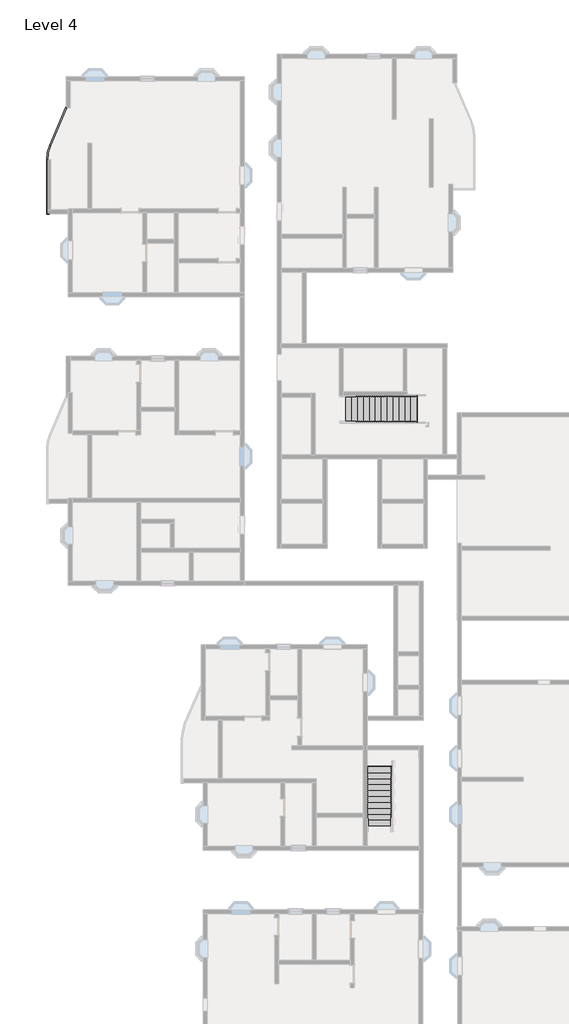
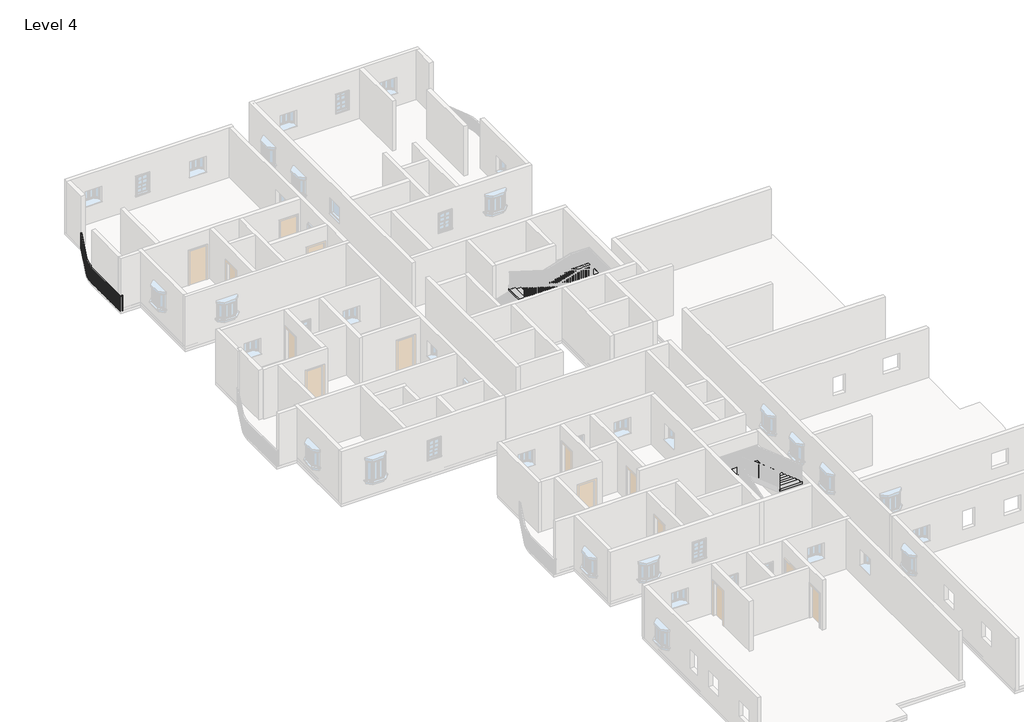
# One storey, part 12 of 14: 2 stair flights, 1 railing.
"""IFC4 building model written with IfcOpenShell, lengths in millimetres."""

from ifc_helpers import new_model, si_unit, frame, origin, place, context, project, spatial, polyline, circle_curve, outline, extrude, transform, mapped, element, save
from ifc_brep_helpers import plane_surface, cylinder_surface, revolved_surface, advanced_brep
from components import stair_flight_ff411a25, stair_flight_aa8d9d08

model = new_model("IFC4")

# Units and contexts
model_context = context("Model", 3, world=origin())
ifc_project = project(units=[si_unit("LENGTHUNIT", "METRE", prefix="MILLI")], contexts=[model_context])

# Site, building, storey
site = spatial("IfcSite", under=ifc_project)
building = spatial("IfcBuilding", under=site)
storey = spatial("IfcBuildingStorey", under=building, Name="Level 4", Elevation=9144.0)

# Railing
placement = place(None, origin())
element("IfcRailing", 1, ObjectType="Handrail - Rectangular", at=placement, inside=storey, context=model_context, shape_type="SolidModel", body=[
    advanced_brep(
    [(-19327.739878, 27355.8257339, 10058.4), (-19327.739878, 27355.8257339, 10007.6), (-19374.4383922, 27375.822953, 10007.6), (-19374.4383922, 27375.822953, 10058.4), (-20162.483418, 25406.4905323, 10058.4), (-20162.483418, 25406.4905323, 10007.6), (-20209.1819322, 25426.4877514, 10007.6), (-20209.1819322, 25426.4877514, 10058.4), (-20316.2891351, 24656.5948172, 10007.6), (-20316.2891351, 24656.5948172, 10058.4), (-20367.0891351, 24656.5948172, 10007.6), (-20367.0891351, 24656.5948172, 10058.4), (-20316.2891351, 21915.0583494, 10058.4), (-20316.2891351, 21915.0583494, 10007.6), (-20367.0891351, 21864.2583494, 10007.6), (-20367.0891351, 21864.2583494, 10058.4), (-20240.0891351, 21915.0583494, 10058.4), (-20240.0891351, 21864.2583494, 10058.4), (-20240.0891351, 21864.2583494, 10007.6), (-20240.0891351, 21915.0583494, 10007.6)],
    [
        (0, 1),
        (1, 2),
        (2, 3),
        (3, 0),
        (0, 4),
        (4, 5),
        (5, 1),
        (5, 6),
        (6, 2),
        (6, 7),
        (7, 3),
        (7, 4),
        (8, 5, circle_curve(frame((-18411.2891351, 24656.5948172, 10007.6), z_axis=(0.0, 0.0, -1.0), x_axis=(-0.9192620907623792, 0.3936460446736121, 0.0)), 1905.0)),
        (4, 9, circle_curve(frame((-18411.2891351, 24656.5948172, 10058.4), z_axis=(0.0, 0.0, 1.0), x_axis=(-0.9192620907623792, 0.3936460446736121, 0.0)), 1905.0)),
        (9, 8),
        (10, 6, circle_curve(frame((-18411.2891351, 24656.5948172, 10007.6), z_axis=(0.0, 0.0, -1.0), x_axis=(-0.9192620907623792, 0.3936460446736121, 0.0)), 1955.8)),
        (8, 10),
        (11, 7, circle_curve(frame((-18411.2891351, 24656.5948172, 10058.4), z_axis=(0.0, 0.0, -1.0), x_axis=(-0.9192620907623792, 0.3936460446736121, 0.0)), 1955.8)),
        (10, 11),
        (11, 9),
        (9, 12),
        (12, 13),
        (13, 8),
        (13, 14),
        (14, 10),
        (14, 15),
        (15, 11),
        (15, 12),
        (16, 17),
        (17, 18),
        (18, 19),
        (19, 16),
        (12, 16),
        (19, 13),
        (18, 14),
        (17, 15),
    ],
    [
        plane_surface(frame((-19351.0891351, 27365.8243434, 10058.4), z_axis=(0.3936460446736102, 0.91926209076238, 0.0), x_axis=(0.91926209076238, -0.3936460446736102, 0.0))),
        plane_surface(frame((-19327.739878, 27355.8257339, 10058.4), z_axis=(0.91926209076238, -0.3936460446736102, 0.0), x_axis=(-0.3936460446736102, -0.91926209076238, 0.0))),
        plane_surface(frame((-19327.739878, 27355.8257339, 10007.6), z_axis=(0.0, 0.0, -1.0), x_axis=(-0.3936460446736102, -0.91926209076238, 0.0))),
        plane_surface(frame((-19374.4383922, 27375.822953, 10007.6), z_axis=(-0.91926209076238, 0.3936460446736102, 0.0), x_axis=(-0.3936460446736102, -0.91926209076238, 0.0))),
        plane_surface(frame((-19374.4383922, 27375.822953, 10058.4), z_axis=(0.0, 0.0, 1.0), x_axis=(-0.3936460446736102, -0.91926209076238, 0.0))),
        revolved_surface(polyline([(-20162.48341800233, 25406.49053230323, 10058.4), (-20162.48341800233, 25406.49053230323, 10007.6)]), (-18411.2891351, 24656.5948172, 10058.4), (0.0, 0.0, 1.0)),
        plane_surface(frame((-18411.2891351, 24656.5948172, 10007.6), z_axis=(0.0, 0.0, -1.0), x_axis=(-0.9192620907623792, 0.3936460446736121, 0.0))),
        cylinder_surface(frame((-18411.2891351, 24656.5948172, 10058.4), z_axis=(0.0, 0.0, 1.0), x_axis=(-0.9192620907623792, 0.3936460446736121, 0.0)), 1955.8),
        plane_surface(frame((-18411.2891351, 24656.5948172, 10058.4), z_axis=(0.0, 0.0, 1.0), x_axis=(-0.9192620907623792, 0.3936460446736121, 0.0))),
        plane_surface(frame((-20316.2891351, 24656.5948172, 10058.4), z_axis=(1.0, 0.0, 0.0), x_axis=(0.0, -1.0, 0.0))),
        plane_surface(frame((-20316.2891351, 24656.5948172, 10007.6), z_axis=(0.0, 0.0, -1.0), x_axis=(0.0, -1.0, 0.0))),
        plane_surface(frame((-20367.0891351, 24656.5948172, 10007.6), z_axis=(-1.0, 0.0, 0.0), x_axis=(0.0, -1.0, 0.0))),
        plane_surface(frame((-20367.0891351, 24656.5948172, 10058.4), z_axis=(0.0, 0.0, 1.0), x_axis=(0.0, -1.0, 0.0))),
        plane_surface(frame((-20240.0891351, 21889.6583494, 10058.4), z_axis=(1.0, 0.0, 0.0), x_axis=(0.0, 1.0, 0.0))),
        plane_surface(frame((-20316.2891351, 21915.0583494, 10058.4), z_axis=(0.0, 1.0, 0.0), x_axis=(1.0, 0.0, 0.0))),
        plane_surface(frame((-20316.2891351, 21915.0583494, 10007.6), z_axis=(0.0, 0.0, -1.0), x_axis=(1.0, 0.0, 0.0))),
        plane_surface(frame((-20367.0891351, 21864.2583494, 10007.6), z_axis=(0.0, -1.0, 0.0), x_axis=(1.0, 0.0, 0.0))),
        plane_surface(frame((-20367.0891351, 21864.2583494, 10058.4), z_axis=(0.0, 0.0, 1.0), x_axis=(1.0, 0.0, 0.0))),
    ],
    [
        (0, [[1, 2, 3, 4]]),
        (1, [[-1, 5, 6, 7]]),
        (2, [[-2, -7, 8, 9]]),
        (3, [[-3, -9, 10, 11]]),
        (4, [[-4, -11, 12, -5]]),
        (5, [[13, -6, 14, 15]]),
        (6, [[16, -8, -13, 17]]),
        (7, [[18, -10, -16, 19]]),
        (8, [[-14, -12, -18, 20]]),
        (9, [[-15, 21, 22, 23]]),
        (10, [[-17, -23, 24, 25]]),
        (11, [[-19, -25, 26, 27]]),
        (12, [[-20, -27, 28, -21]]),
        (13, [[29, 30, 31, 32]]),
        (14, [[-22, 33, -32, 34]]),
        (15, [[-24, -34, -31, 35]]),
        (16, [[-26, -35, -30, 36]]),
        (17, [[-28, -36, -29, -33]]),
    ],
),
    extrude(outline(polyline([(-20351.2141351, 21922.9198172), (-20332.1641351, 21922.9198172), (-20332.1641351, 21903.8698172), (-20351.2141351, 21903.8698172), (-20351.2141351, 21922.9198172)])), frame((0.0, 0.0, 9144.0), z_axis=(0.0, 0.0, 1.0), x_axis=(1.0, 0.0, 0.0)), (0.0, 0.0, 1.0), 863.6),
    extrude(outline(polyline([(-20351.2141351, 22024.5198172), (-20332.1641351, 22024.5198172), (-20332.1641351, 22005.4698172), (-20351.2141351, 22005.4698172), (-20351.2141351, 22024.5198172)])), frame((0.0, 0.0, 9144.0), z_axis=(0.0, 0.0, 1.0), x_axis=(1.0, 0.0, 0.0)), (0.0, 0.0, 1.0), 863.6),
    extrude(outline(polyline([(-20351.2141351, 22126.1198172), (-20332.1641351, 22126.1198172), (-20332.1641351, 22107.0698172), (-20351.2141351, 22107.0698172), (-20351.2141351, 22126.1198172)])), frame((0.0, 0.0, 9144.0), z_axis=(0.0, 0.0, 1.0), x_axis=(1.0, 0.0, 0.0)), (0.0, 0.0, 1.0), 863.6),
    extrude(outline(polyline([(-20351.2141351, 22227.7198172), (-20332.1641351, 22227.7198172), (-20332.1641351, 22208.6698172), (-20351.2141351, 22208.6698172), (-20351.2141351, 22227.7198172)])), frame((0.0, 0.0, 9144.0), z_axis=(0.0, 0.0, 1.0), x_axis=(1.0, 0.0, 0.0)), (0.0, 0.0, 1.0), 863.6),
    extrude(outline(polyline([(-20351.2141351, 22329.3198172), (-20332.1641351, 22329.3198172), (-20332.1641351, 22310.2698172), (-20351.2141351, 22310.2698172), (-20351.2141351, 22329.3198172)])), frame((0.0, 0.0, 9144.0), z_axis=(0.0, 0.0, 1.0), x_axis=(1.0, 0.0, 0.0)), (0.0, 0.0, 1.0), 863.6),
    extrude(outline(polyline([(-20351.2141351, 22430.9198172), (-20332.1641351, 22430.9198172), (-20332.1641351, 22411.8698172), (-20351.2141351, 22411.8698172), (-20351.2141351, 22430.9198172)])), frame((0.0, 0.0, 9144.0), z_axis=(0.0, 0.0, 1.0), x_axis=(1.0, 0.0, 0.0)), (0.0, 0.0, 1.0), 863.6),
    extrude(outline(polyline([(-20351.2141351, 22532.5198172), (-20332.1641351, 22532.5198172), (-20332.1641351, 22513.4698172), (-20351.2141351, 22513.4698172), (-20351.2141351, 22532.5198172)])), frame((0.0, 0.0, 9144.0), z_axis=(0.0, 0.0, 1.0), x_axis=(1.0, 0.0, 0.0)), (0.0, 0.0, 1.0), 863.6),
    extrude(outline(polyline([(-20351.2141351, 22634.1198172), (-20332.1641351, 22634.1198172), (-20332.1641351, 22615.0698172), (-20351.2141351, 22615.0698172), (-20351.2141351, 22634.1198172)])), frame((0.0, 0.0, 9144.0), z_axis=(0.0, 0.0, 1.0), x_axis=(1.0, 0.0, 0.0)), (0.0, 0.0, 1.0), 863.6),
    extrude(outline(polyline([(-20351.2141351, 22735.7198172), (-20332.1641351, 22735.7198172), (-20332.1641351, 22716.6698172), (-20351.2141351, 22716.6698172), (-20351.2141351, 22735.7198172)])), frame((0.0, 0.0, 9144.0), z_axis=(0.0, 0.0, 1.0), x_axis=(1.0, 0.0, 0.0)), (0.0, 0.0, 1.0), 863.6),
    extrude(outline(polyline([(-20351.2141351, 22837.3198172), (-20332.1641351, 22837.3198172), (-20332.1641351, 22818.2698172), (-20351.2141351, 22818.2698172), (-20351.2141351, 22837.3198172)])), frame((0.0, 0.0, 9144.0), z_axis=(0.0, 0.0, 1.0), x_axis=(1.0, 0.0, 0.0)), (0.0, 0.0, 1.0), 863.6),
    extrude(outline(polyline([(-20351.2141351, 22938.9198172), (-20332.1641351, 22938.9198172), (-20332.1641351, 22919.8698172), (-20351.2141351, 22919.8698172), (-20351.2141351, 22938.9198172)])), frame((0.0, 0.0, 9144.0), z_axis=(0.0, 0.0, 1.0), x_axis=(1.0, 0.0, 0.0)), (0.0, 0.0, 1.0), 863.6),
    extrude(outline(polyline([(-20351.2141351, 23040.5198172), (-20332.1641351, 23040.5198172), (-20332.1641351, 23021.4698172), (-20351.2141351, 23021.4698172), (-20351.2141351, 23040.5198172)])), frame((0.0, 0.0, 9144.0), z_axis=(0.0, 0.0, 1.0), x_axis=(1.0, 0.0, 0.0)), (0.0, 0.0, 1.0), 863.6),
    extrude(outline(polyline([(-20351.2141351, 23142.1198172), (-20332.1641351, 23142.1198172), (-20332.1641351, 23123.0698172), (-20351.2141351, 23123.0698172), (-20351.2141351, 23142.1198172)])), frame((0.0, 0.0, 9144.0), z_axis=(0.0, 0.0, 1.0), x_axis=(1.0, 0.0, 0.0)), (0.0, 0.0, 1.0), 863.6),
    extrude(outline(polyline([(-20351.2141351, 23243.7198172), (-20332.1641351, 23243.7198172), (-20332.1641351, 23224.6698172), (-20351.2141351, 23224.6698172), (-20351.2141351, 23243.7198172)])), frame((0.0, 0.0, 9144.0), z_axis=(0.0, 0.0, 1.0), x_axis=(1.0, 0.0, 0.0)), (0.0, 0.0, 1.0), 863.6),
    extrude(outline(polyline([(-20351.2141351, 23345.3198172), (-20332.1641351, 23345.3198172), (-20332.1641351, 23326.2698172), (-20351.2141351, 23326.2698172), (-20351.2141351, 23345.3198172)])), frame((0.0, 0.0, 9144.0), z_axis=(0.0, 0.0, 1.0), x_axis=(1.0, 0.0, 0.0)), (0.0, 0.0, 1.0), 863.6),
    extrude(outline(polyline([(-20351.2141351, 23446.9198172), (-20332.1641351, 23446.9198172), (-20332.1641351, 23427.8698172), (-20351.2141351, 23427.8698172), (-20351.2141351, 23446.9198172)])), frame((0.0, 0.0, 9144.0), z_axis=(0.0, 0.0, 1.0), x_axis=(1.0, 0.0, 0.0)), (0.0, 0.0, 1.0), 863.6),
    extrude(outline(polyline([(-20351.2141351, 23548.5198172), (-20332.1641351, 23548.5198172), (-20332.1641351, 23529.4698172), (-20351.2141351, 23529.4698172), (-20351.2141351, 23548.5198172)])), frame((0.0, 0.0, 9144.0), z_axis=(0.0, 0.0, 1.0), x_axis=(1.0, 0.0, 0.0)), (0.0, 0.0, 1.0), 863.6),
    extrude(outline(polyline([(-20351.2141351, 23650.1198172), (-20332.1641351, 23650.1198172), (-20332.1641351, 23631.0698172), (-20351.2141351, 23631.0698172), (-20351.2141351, 23650.1198172)])), frame((0.0, 0.0, 9144.0), z_axis=(0.0, 0.0, 1.0), x_axis=(1.0, 0.0, 0.0)), (0.0, 0.0, 1.0), 863.6),
    extrude(outline(polyline([(-20351.2141351, 23751.7198172), (-20332.1641351, 23751.7198172), (-20332.1641351, 23732.6698172), (-20351.2141351, 23732.6698172), (-20351.2141351, 23751.7198172)])), frame((0.0, 0.0, 9144.0), z_axis=(0.0, 0.0, 1.0), x_axis=(1.0, 0.0, 0.0)), (0.0, 0.0, 1.0), 863.6),
    extrude(outline(polyline([(-20351.2141351, 23853.3198172), (-20332.1641351, 23853.3198172), (-20332.1641351, 23834.2698172), (-20351.2141351, 23834.2698172), (-20351.2141351, 23853.3198172)])), frame((0.0, 0.0, 9144.0), z_axis=(0.0, 0.0, 1.0), x_axis=(1.0, 0.0, 0.0)), (0.0, 0.0, 1.0), 863.6),
    extrude(outline(polyline([(-20351.2141351, 23954.9198172), (-20332.1641351, 23954.9198172), (-20332.1641351, 23935.8698172), (-20351.2141351, 23935.8698172), (-20351.2141351, 23954.9198172)])), frame((0.0, 0.0, 9144.0), z_axis=(0.0, 0.0, 1.0), x_axis=(1.0, 0.0, 0.0)), (0.0, 0.0, 1.0), 863.6),
    extrude(outline(polyline([(-20351.2141351, 24056.5198172), (-20332.1641351, 24056.5198172), (-20332.1641351, 24037.4698172), (-20351.2141351, 24037.4698172), (-20351.2141351, 24056.5198172)])), frame((0.0, 0.0, 9144.0), z_axis=(0.0, 0.0, 1.0), x_axis=(1.0, 0.0, 0.0)), (0.0, 0.0, 1.0), 863.6),
    extrude(outline(polyline([(-20351.2141351, 24158.1198172), (-20332.1641351, 24158.1198172), (-20332.1641351, 24139.0698172), (-20351.2141351, 24139.0698172), (-20351.2141351, 24158.1198172)])), frame((0.0, 0.0, 9144.0), z_axis=(0.0, 0.0, 1.0), x_axis=(1.0, 0.0, 0.0)), (0.0, 0.0, 1.0), 863.6),
    extrude(outline(polyline([(-20351.2141351, 24259.7198172), (-20332.1641351, 24259.7198172), (-20332.1641351, 24240.6698172), (-20351.2141351, 24240.6698172), (-20351.2141351, 24259.7198172)])), frame((0.0, 0.0, 9144.0), z_axis=(0.0, 0.0, 1.0), x_axis=(1.0, 0.0, 0.0)), (0.0, 0.0, 1.0), 863.6),
    extrude(outline(polyline([(-20351.2141351, 24361.3198172), (-20332.1641351, 24361.3198172), (-20332.1641351, 24342.2698172), (-20351.2141351, 24342.2698172), (-20351.2141351, 24361.3198172)])), frame((0.0, 0.0, 9144.0), z_axis=(0.0, 0.0, 1.0), x_axis=(1.0, 0.0, 0.0)), (0.0, 0.0, 1.0), 863.6),
    extrude(outline(polyline([(-20351.2141351, 24462.9198172), (-20332.1641351, 24462.9198172), (-20332.1641351, 24443.8698172), (-20351.2141351, 24443.8698172), (-20351.2141351, 24462.9198172)])), frame((0.0, 0.0, 9144.0), z_axis=(0.0, 0.0, 1.0), x_axis=(1.0, 0.0, 0.0)), (0.0, 0.0, 1.0), 863.6),
    extrude(outline(polyline([(-20351.2141351, 24564.5198172), (-20332.1641351, 24564.5198172), (-20332.1641351, 24545.4698172), (-20351.2141351, 24545.4698172), (-20351.2141351, 24564.5198172)])), frame((0.0, 0.0, 9144.0), z_axis=(0.0, 0.0, 1.0), x_axis=(1.0, 0.0, 0.0)), (0.0, 0.0, 1.0), 863.6),
    extrude(outline(polyline([(-20349.6005818, 24736.2720848), (-20330.5630441, 24735.5831307), (-20331.2519982, 24716.545593), (-20350.289536, 24717.2345471), (-20349.6005818, 24736.2720848)])), frame((0.0, 0.0, 9144.0), z_axis=(0.0, 0.0, 1.0), x_axis=(1.0, 0.0, 0.0)), (0.0, 0.0, 1.0), 863.6),
    extrude(outline(polyline([(-20342.724955, 24838.1310534), (-20323.750023, 24836.4415402), (-20325.4395363, 24817.4666081), (-20344.4144683, 24819.1561214), (-20342.724955, 24838.1310534)])), frame((0.0, 0.0, 9144.0), z_axis=(0.0, 0.0, 1.0), x_axis=(1.0, 0.0, 0.0)), (0.0, 0.0, 1.0), 863.6),
    extrude(outline(polyline([(-20330.5003254, 24939.4872677), (-20311.6405491, 24936.8018743), (-20314.3259425, 24917.942098), (-20333.1857188, 24920.6274914), (-20330.5003254, 24939.4872677)])), frame((0.0, 0.0, 9144.0), z_axis=(0.0, 0.0, 1.0), x_axis=(1.0, 0.0, 0.0)), (0.0, 0.0, 1.0), 863.6),
    extrude(outline(polyline([(-20312.9605484, 25040.0600272), (-20294.2681589, 25036.3861907), (-20297.9419954, 25017.6938012), (-20316.6343849, 25021.3676377), (-20312.9605484, 25040.0600272)])), frame((0.0, 0.0, 9144.0), z_axis=(0.0, 0.0, 1.0), x_axis=(1.0, 0.0, 0.0)), (0.0, 0.0, 1.0), 863.6),
    extrude(outline(polyline([(-20290.1541995, 25139.5708014), (-20271.6809643, 25134.9186963), (-20276.3330693, 25116.4454611), (-20294.8063045, 25121.0975662), (-20290.1541995, 25139.5708014)])), frame((0.0, 0.0, 9144.0), z_axis=(0.0, 0.0, 1.0), x_axis=(1.0, 0.0, 0.0)), (0.0, 0.0, 1.0), 863.6),
    extrude(outline(polyline([(-20262.1444395, 25237.7440008), (-20243.9415192, 25232.1265109), (-20249.5590091, 25213.9235906), (-20267.7619294, 25219.5410805), (-20262.1444395, 25237.7440008)])), frame((0.0, 0.0, 9144.0), z_axis=(0.0, 0.0, 1.0), x_axis=(1.0, 0.0, 0.0)), (0.0, 0.0, 1.0), 863.6),
    extrude(outline(polyline([(-20229.0088399, 25334.3077402), (-20211.1266465, 25327.7404228), (-20217.693964, 25309.8582293), (-20235.5761574, 25316.4255468), (-20229.0088399, 25334.3077402)])), frame((0.0, 0.0, 9144.0), z_axis=(0.0, 0.0, 1.0), x_axis=(1.0, 0.0, 0.0)), (0.0, 0.0, 1.0), 863.6),
    extrude(outline(polyline([(-20155.9843907, 25510.389225), (-20138.4724479, 25502.8902678), (-20145.9714051, 25485.378325), (-20163.4833479, 25492.8772822), (-20155.9843907, 25510.389225)])), frame((0.0, 0.0, 9144.0), z_axis=(0.0, 0.0, 1.0), x_axis=(1.0, 0.0, 0.0)), (0.0, 0.0, 1.0), 863.6),
    extrude(outline(polyline([(-20115.9899526, 25603.7862534), (-20098.4780098, 25596.2872963), (-20105.9769669, 25578.7753534), (-20123.4889098, 25586.2743106), (-20115.9899526, 25603.7862534)])), frame((0.0, 0.0, 9144.0), z_axis=(0.0, 0.0, 1.0), x_axis=(1.0, 0.0, 0.0)), (0.0, 0.0, 1.0), 863.6),
    extrude(outline(polyline([(-20075.9955145, 25697.1832818), (-20058.4835716, 25689.6843247), (-20065.9825288, 25672.1723818), (-20083.4944716, 25679.671339), (-20075.9955145, 25697.1832818)])), frame((0.0, 0.0, 9144.0), z_axis=(0.0, 0.0, 1.0), x_axis=(1.0, 0.0, 0.0)), (0.0, 0.0, 1.0), 863.6),
    extrude(outline(polyline([(-20036.0010763, 25790.5803103), (-20018.4891335, 25783.0813531), (-20025.9880906, 25765.5694103), (-20043.5000335, 25773.0683674), (-20036.0010763, 25790.5803103)])), frame((0.0, 0.0, 9144.0), z_axis=(0.0, 0.0, 1.0), x_axis=(1.0, 0.0, 0.0)), (0.0, 0.0, 1.0), 863.6),
    extrude(outline(polyline([(-19996.0066382, 25883.9773387), (-19978.4946954, 25876.4783815), (-19985.9936525, 25858.9664387), (-20003.5055953, 25866.4653958), (-19996.0066382, 25883.9773387)])), frame((0.0, 0.0, 9144.0), z_axis=(0.0, 0.0, 1.0), x_axis=(1.0, 0.0, 0.0)), (0.0, 0.0, 1.0), 863.6),
    extrude(outline(polyline([(-19956.0122, 25977.3743671), (-19938.5002572, 25969.8754099), (-19945.9992144, 25952.3634671), (-19963.5111572, 25959.8624243), (-19956.0122, 25977.3743671)])), frame((0.0, 0.0, 9144.0), z_axis=(0.0, 0.0, 1.0), x_axis=(1.0, 0.0, 0.0)), (0.0, 0.0, 1.0), 863.6),
    extrude(outline(polyline([(-19916.0177619, 26070.7713955), (-19898.5058191, 26063.2724384), (-19906.0047762, 26045.7604955), (-19923.5167191, 26053.2594527), (-19916.0177619, 26070.7713955)])), frame((0.0, 0.0, 9144.0), z_axis=(0.0, 0.0, 1.0), x_axis=(1.0, 0.0, 0.0)), (0.0, 0.0, 1.0), 863.6),
    extrude(outline(polyline([(-19876.0233238, 26164.1684239), (-19858.5113809, 26156.6694668), (-19866.0103381, 26139.157524), (-19883.5222809, 26146.6564811), (-19876.0233238, 26164.1684239)])), frame((0.0, 0.0, 9144.0), z_axis=(0.0, 0.0, 1.0), x_axis=(1.0, 0.0, 0.0)), (0.0, 0.0, 1.0), 863.6),
    extrude(outline(polyline([(-19836.0288856, 26257.5654524), (-19818.5169428, 26250.0664952), (-19826.0159, 26232.5545524), (-19843.5278428, 26240.0535095), (-19836.0288856, 26257.5654524)])), frame((0.0, 0.0, 9144.0), z_axis=(0.0, 0.0, 1.0), x_axis=(1.0, 0.0, 0.0)), (0.0, 0.0, 1.0), 863.6),
    extrude(outline(polyline([(-19796.0344475, 26350.9624808), (-19778.5225047, 26343.4635236), (-19786.0214618, 26325.9515808), (-19803.5334046, 26333.450538), (-19796.0344475, 26350.9624808)])), frame((0.0, 0.0, 9144.0), z_axis=(0.0, 0.0, 1.0), x_axis=(1.0, 0.0, 0.0)), (0.0, 0.0, 1.0), 863.6),
    extrude(outline(polyline([(-19756.0400094, 26444.3595092), (-19738.5280665, 26436.860552), (-19746.0270237, 26419.3486092), (-19763.5389665, 26426.8475664), (-19756.0400094, 26444.3595092)])), frame((0.0, 0.0, 9144.0), z_axis=(0.0, 0.0, 1.0), x_axis=(1.0, 0.0, 0.0)), (0.0, 0.0, 1.0), 863.6),
    extrude(outline(polyline([(-19716.0455712, 26537.7565376), (-19698.5336284, 26530.2575805), (-19706.0325855, 26512.7456376), (-19723.5445284, 26520.2445948), (-19716.0455712, 26537.7565376)])), frame((0.0, 0.0, 9144.0), z_axis=(0.0, 0.0, 1.0), x_axis=(1.0, 0.0, 0.0)), (0.0, 0.0, 1.0), 863.6),
    extrude(outline(polyline([(-19676.0511331, 26631.153566), (-19658.5391902, 26623.6546089), (-19666.0381474, 26606.1426661), (-19683.5500902, 26613.6416232), (-19676.0511331, 26631.153566)])), frame((0.0, 0.0, 9144.0), z_axis=(0.0, 0.0, 1.0), x_axis=(1.0, 0.0, 0.0)), (0.0, 0.0, 1.0), 863.6),
    extrude(outline(polyline([(-19636.0566949, 26724.5505945), (-19618.5447521, 26717.0516373), (-19626.0437093, 26699.5396945), (-19643.5556521, 26707.0386516), (-19636.0566949, 26724.5505945)])), frame((0.0, 0.0, 9144.0), z_axis=(0.0, 0.0, 1.0), x_axis=(1.0, 0.0, 0.0)), (0.0, 0.0, 1.0), 863.6),
    extrude(outline(polyline([(-19596.0622568, 26817.9476229), (-19578.550314, 26810.4486657), (-19586.0492711, 26792.9367229), (-19603.561214, 26800.4356801), (-19596.0622568, 26817.9476229)])), frame((0.0, 0.0, 9144.0), z_axis=(0.0, 0.0, 1.0), x_axis=(1.0, 0.0, 0.0)), (0.0, 0.0, 1.0), 863.6),
    extrude(outline(polyline([(-19556.0678187, 26911.3446513), (-19538.5558758, 26903.8456942), (-19546.054833, 26886.3337513), (-19563.5667758, 26893.8327085), (-19556.0678187, 26911.3446513)])), frame((0.0, 0.0, 9144.0), z_axis=(0.0, 0.0, 1.0), x_axis=(1.0, 0.0, 0.0)), (0.0, 0.0, 1.0), 863.6),
    extrude(outline(polyline([(-19516.0733805, 27004.7416797), (-19498.5614377, 26997.2427226), (-19506.0603948, 26979.7307797), (-19523.5723377, 26987.2297369), (-19516.0733805, 27004.7416797)])), frame((0.0, 0.0, 9144.0), z_axis=(0.0, 0.0, 1.0), x_axis=(1.0, 0.0, 0.0)), (0.0, 0.0, 1.0), 863.6),
    extrude(outline(polyline([(-19476.0789424, 27098.1387082), (-19458.5669996, 27090.639751), (-19466.0659567, 27073.1278082), (-19483.5778995, 27080.6267653), (-19476.0789424, 27098.1387082)])), frame((0.0, 0.0, 9144.0), z_axis=(0.0, 0.0, 1.0), x_axis=(1.0, 0.0, 0.0)), (0.0, 0.0, 1.0), 863.6),
    extrude(outline(polyline([(-19436.0845042, 27191.5357366), (-19418.5725614, 27184.0367794), (-19426.0715186, 27166.5248366), (-19443.5834614, 27174.0237937), (-19436.0845042, 27191.5357366)])), frame((0.0, 0.0, 9144.0), z_axis=(0.0, 0.0, 1.0), x_axis=(1.0, 0.0, 0.0)), (0.0, 0.0, 1.0), 863.6),
    extrude(outline(polyline([(-19396.0900661, 27284.932765), (-19378.5781233, 27277.4338078), (-19386.0770804, 27259.921865), (-19403.5890233, 27267.4208222), (-19396.0900661, 27284.932765)])), frame((0.0, 0.0, 9144.0), z_axis=(0.0, 0.0, 1.0), x_axis=(1.0, 0.0, 0.0)), (0.0, 0.0, 1.0), 863.6),
    extrude(outline(polyline([(-20351.2141351, 21899.1833494), (-20332.1641351, 21899.1833494), (-20332.1641351, 21880.1333494), (-20351.2141351, 21880.1333494), (-20351.2141351, 21899.1833494)])), frame((0.0, 0.0, 9144.0), z_axis=(0.0, 0.0, 1.0), x_axis=(1.0, 0.0, 0.0)), (0.0, 0.0, 1.0), 863.6),
    extrude(outline(polyline([(-20351.2141351, 24666.1198172), (-20332.1641351, 24666.1198172), (-20332.1641351, 24647.0698172), (-20351.2141351, 24647.0698172), (-20351.2141351, 24666.1198172)])), frame((0.0, 0.0, 9144.0), z_axis=(0.0, 0.0, 1.0), x_axis=(1.0, 0.0, 0.0)), (0.0, 0.0, 1.0), 863.6),
    extrude(outline(polyline([(-20190.839168, 25428.9945919), (-20173.3272251, 25421.4956347), (-20180.8261823, 25403.9836919), (-20198.3381251, 25411.482649), (-20190.839168, 25428.9945919)])), frame((0.0, 0.0, 9144.0), z_axis=(0.0, 0.0, 1.0), x_axis=(1.0, 0.0, 0.0)), (0.0, 0.0, 1.0), 863.6),
    extrude(outline(polyline([(-20259.1391351, 21880.1333494), (-20259.1391351, 21899.1833494), (-20240.0891351, 21899.1833494), (-20240.0891351, 21880.1333494), (-20259.1391351, 21880.1333494)])), frame((0.0, 0.0, 9144.0), z_axis=(0.0, 0.0, 1.0), x_axis=(1.0, 0.0, 0.0)), (0.0, 0.0, 1.0), 863.6),
    extrude(outline(polyline([(-19359.8451065, 27369.573822), (-19342.3331637, 27362.0748648), (-19349.8321209, 27344.562922), (-19367.3440637, 27352.0618792), (-19359.8451065, 27369.573822)])), frame((0.0, 0.0, 9144.0), z_axis=(0.0, 0.0, 1.0), x_axis=(1.0, 0.0, 0.0)), (0.0, 0.0, 1.0), 863.6),
])

# Stair flights
stair_flight_shape = stair_flight_ff411a25(model_context)
element("IfcStairFlight", 2, ObjectType="2\" Tread 1\" Nosing 1/4\" Riser", at=placement, inside=storey, context=model_context, shape_type="MappedRepresentation", body=[
    mapped(stair_flight_shape, transform((0.0, 0.0, 0.0), x_axis=(1.0, 0.0, 0.0), y_axis=(0.0, 1.0, 0.0), z_axis=(0.0, 0.0, 1.0))),
])
stair_flight_2_shape = stair_flight_aa8d9d08(model_context)
element("IfcStairFlight", 3, ObjectType="2\" Tread 1\" Nosing 1/4\" Riser", at=placement, inside=storey, context=model_context, shape_type="MappedRepresentation", body=[
    mapped(stair_flight_2_shape, transform((0.0, 0.0, 0.0), x_axis=(1.0, 0.0, 0.0), y_axis=(0.0, 1.0, 0.0), z_axis=(0.0, 0.0, 1.0))),
])

save(model, "model.ifc")

# Revit data of these elements
# Type "Handrail - Rectangular"
#   Assembly Code = "C2010400"
#   built-in parameter 1008612 = 0.0416667 (stored number, unit not read)
#   built-in parameter 1008611 = 0.0416667 (stored number, unit not read)
#   built-in parameter 1008609 = 0.333333 (stored number, unit not read)
#   built-in parameter 1008604 = 0.166667 (stored number, unit not read)
#   built-in parameter 1008603 = 0.166667 (stored number, unit not read)
#   Railing Height = 3' - 0"
#   built-in parameter 1008630 = 2
#   built-in parameter 1008610 = 2
#   built-in parameter 1008618 = Baluster - Square : 3/4"
# Element 1 (IfcRailing, "Handrail - Rectangular")
#   Phase Created = New Construction
# Elements 2, 3 (IfcStairFlight, "2\" Tread 1\" Nosing 1/4\" Riser")
#   Phase Created = New Construction
